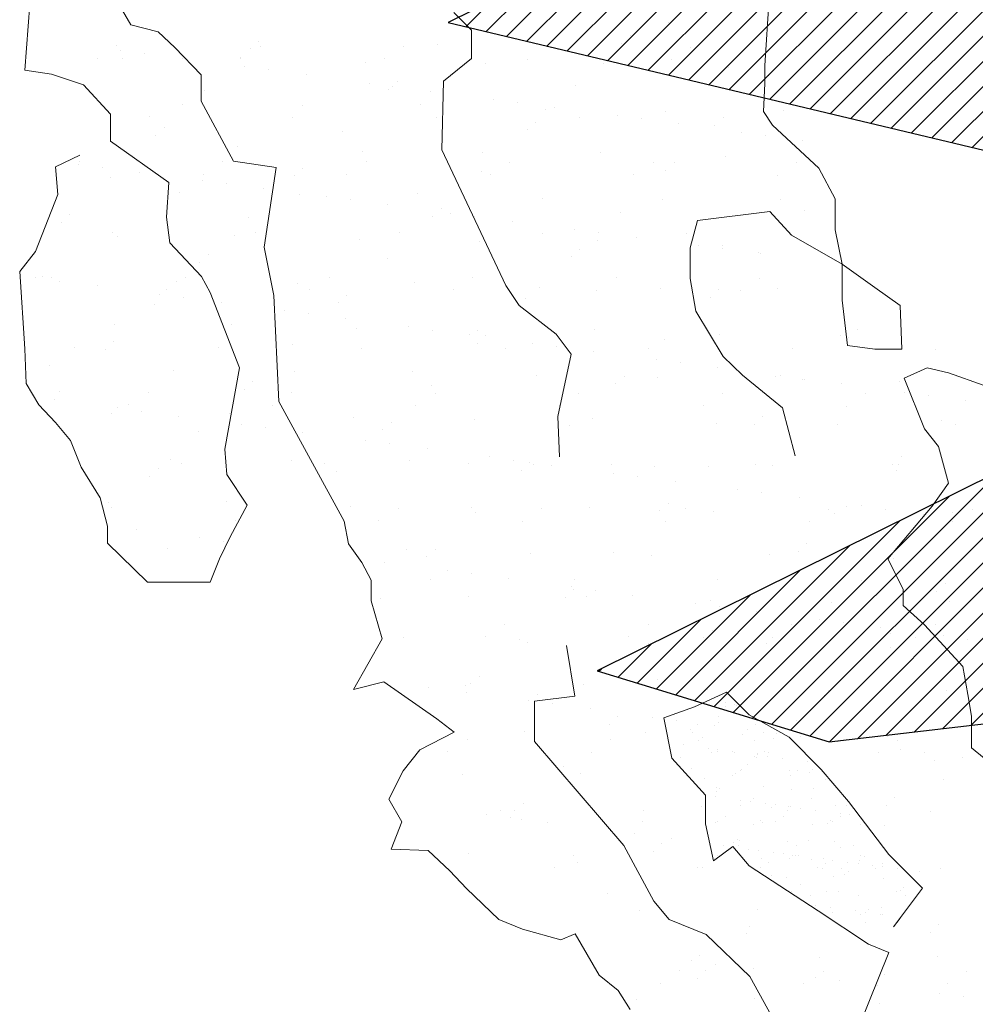
# Model space of a CAD drawing. Units: inches. Extents: x 1986 to 21484, y -1816 to 2016.
# Tile 14 of 85: x 2149.949 to 2158.236, y 1873.899 to 1882.437. Entities that reach past the tile are written whole.
import ezdxf

# ---------------------------------------------------------------- set-up
doc = ezdxf.new("R2010")
doc.units = ezdxf.units.IN
doc.layers.add('L-PLNT', color=84, linetype='Continuous', lineweight=13)
doc.layers.add('vfolhas', color=114, linetype='Continuous', lineweight=5)
doc.layers.add('vfolha2', color=110, linetype='Continuous')
doc.layers.add('vfolhas2', color=102, linetype='Continuous')
pattern_1 = [(45, (-2446.5133113, 50.986076), (-0.004419417382, 0.004419417382), [])]

# ---------------------------------------------------------------- blocks, each defined once
blk = doc.blocks.new('arbusto_PB_verde_grande')
at = {"layer": 'vfolha2'}
h = blk.add_hatch(dxfattribs=at)
h.set_pattern_fill('ANSI31', color=256, scale=0.05, style=0)
h.set_pattern_definition(pattern_1)
h.paths.add_polyline_path([(0.02944, 0.35651), (0.00028, 0.09048), (0.02625, -0.03934), (0.047, 0.06233), (0.06189, 0.09731), (0.09372, 0.26573), (0.09955, 0.43473), (0.08789, 0.61313), (0.0645, 0.72266), (0.04988, 0.6851), (0.0236, 0.51294)])
h.paths.add_polyline_path([(0.30106, 0.43789), (0.14225, 0.24871), (0.26685, 0.30022)])
h.paths.add_polyline_path([(0.37995, 0.22817), (0.23697, 0.15193), (0.18428, 0.09364), (0.11122, 0.04358), (0.02625, -0.03934), (0.28061, 0.04667), (0.36829, 0.07798), (0.46756, 0.11239), (0.61068, 0.19376), (0.71585, 0.27823), (0.55813, 0.25948)])
h.paths.add_polyline_path([(0.56101, -0.29441), (0.72752, -0.32573), (0.59024, -0.2412), (0.42962, -0.15982), (0.02625, -0.03934), (0.14922, -0.14107), (0.18838, -0.16604), (0.41501, -0.24435)])
h.paths.add_polyline_path([(-0.27429, -0.44776), (-0.30352, -0.72628), (-0.23923, -0.64175), (-0.15457, -0.45716), (0.02625, -0.03934), (-0.16328, -0.25376)])
h.paths.add_polyline_path([(-0.51963, -0.24744), (-0.67736, -0.32573), (-0.59558, -0.35072), (-0.40574, -0.32882), (-0.21007, -0.20995), (0.02625, -0.03934), (-0.14874, -0.06595), (-0.31518, -0.09101), (-0.41452, -0.15048)])
h.paths.add_polyline_path([(-0.52546, 0.25007), (-0.70947, 0.24698), (-0.51963, 0.1093), (-0.32979, 0.02167), (-0.07567, -0.0128), (-0.04234, -0.02148), (-0.35024, 0.1312)])
at = {"layer": 'vfolhas'}
h = blk.add_hatch(dxfattribs=at)
h.set_pattern_fill('ANSI31', color=256, scale=0.05, style=0)
h.set_pattern_definition(pattern_1)
h.paths.add_polyline_path([(-0.57219, 0.06233), (-0.7153, 0.10298), (-0.67736, 0.08107), (-0.62769, 0.01536), (-0.56347, -0.04095), (-0.26461, -0.0834), (-0.14874, -0.06595), (-0.10151, -0.05877), (-0.20418, -0.0472), (-0.40279, -0.00339)])
h.paths.add_polyline_path([(-0.56347, -0.04095), (-0.58279, -0.02401), (-0.72992, -0.09726), (-0.4334, -0.1679), (-0.41452, -0.15048), (-0.31518, -0.09101), (-0.26461, -0.0834)])
h.paths.add_polyline_path([(-0.2769, -0.47267), (-0.27429, -0.44776), (-0.16328, -0.25376), (0.02625, -0.03934), (-0.21007, -0.20995), (-0.2672, -0.24466), (-0.36485, -0.35697), (-0.42907, -0.46341), (-0.47586, -0.60425), (-0.37946, -0.57603)])
at = {"layer": 'vfolha2'}
for p, q in [((-0.51963, -0.24744), (-0.67736, -0.32573)), ((-0.67736, -0.32573), (-0.59558, -0.35072)), ((-0.59558, -0.35072), (-0.40574, -0.32882))]:
    blk.add_line(p, q, dxfattribs=at)
at = {"layer": 'vfolhas2'}
for p, q in [((-0.58279, -0.02401), (-0.72992, -0.09726)), ((-0.72992, -0.09726), (-0.4334, -0.1679))]:
    blk.add_line(p, q, dxfattribs=at)
blk = doc.blocks.new('PLANT-SHRUB')
for p, q in [((2156.412, 1882.0396), (2156.4637, 1882.8912)), ((2150.0375, 1882.5728), (2149.9922, 1881.9992)), ((2150.9127, 1882.3924), (2150.8403, 1882.5164)), ((2153.8674, 1882.3451), (2153.7137, 1882.4988)), ((2151.1505, 1882.3304), (2150.9127, 1882.3924)), ((2154.5314, 1882.4284), (2154.5314, 1882.4284)), ((2155.5776, 1882.4151), (2155.5776, 1882.4151)), ((2151.2953, 1882.1961), (2151.1505, 1882.3304)), ((2153.8674, 1882.0994), (2153.8674, 1882.3451)), ((2155.2446, 1882.3002), (2155.2446, 1882.3002)), ((2150.7886, 1882.2088), (2150.7886, 1882.2088)), ((2152.0225, 1882.2512), (2152.0225, 1882.2512)), ((2152.0333, 1882.2065), (2152.0333, 1882.2065)), ((2153.5717, 1882.219), (2153.5717, 1882.219)), ((2155.1709, 1882.2327), (2155.1709, 1882.2327)), ((2150.8264, 1882.1709), (2150.8264, 1882.1709)), ((2151.0345, 1882.1435), (2151.0345, 1882.1435)), ((2151.5228, 1881.9584), (2151.2953, 1882.1961)), ((2151.9488, 1882.1836), (2151.9488, 1882.1836)), ((2153.2779, 1882.2043), (2153.2779, 1882.2043)), ((2154.5225, 1882.202), (2154.5225, 1882.202)), ((2155.7672, 1882.1998), (2155.7672, 1882.1998)), ((2150.6201, 1882.1014), (2150.6201, 1882.1014)), ((2150.843, 1882.101), (2150.843, 1882.101)), ((2151.3594, 1882.1007), (2151.3594, 1882.1007)), ((2151.8647, 1882.0992), (2151.8647, 1882.0992)), ((2151.8654, 1882.1059), (2151.8654, 1882.1059)), ((2152.9448, 1882.0671), (2152.9448, 1882.0671)), ((2153.1094, 1882.0969), (2153.1094, 1882.0969)), ((2153.6229, 1881.9049), (2153.8674, 1882.0994)), ((2153.991, 1882.0537), (2153.991, 1882.0537)), ((2154.354, 1882.0946), (2154.354, 1882.0946)), ((2155.0134, 1882.0586), (2155.0134, 1882.0586)), ((2155.5986, 1882.0924), (2155.5986, 1882.0924)), ((2156.412, 1881.8848), (2156.412, 1882.0396)), ((2149.9922, 1881.9992), (2150.2243, 1881.9644)), ((2150.2243, 1881.9644), (2150.5029, 1881.8716)), ((2151.5228, 1881.7311), (2151.5228, 1881.9584)), ((2151.9022, 1882.0292), (2151.9022, 1882.0292)), ((2152.1103, 1882.0018), (2152.1103, 1882.0018)), ((2152.4352, 1881.9591), (2152.4352, 1881.9591)), ((2156.0929, 1882.0197), (2156.0929, 1882.0197)), ((2156.4461, 1881.9494), (2156.4461, 1881.9494)), ((2150.5029, 1881.8716), (2150.7351, 1881.6164)), ((2152.9781, 1881.8876), (2152.9781, 1881.8876)), ((2153.224, 1881.9004), (2153.224, 1881.9004)), ((2153.6083, 1881.3076), (2153.6229, 1881.9049)), ((2153.6229, 1881.9049), (2153.6229, 1881.9049)), ((2154.7731, 1881.8682), (2154.7731, 1881.8682)), ((2156.3724, 1881.8819), (2156.3724, 1881.8819)), ((2156.3991, 1881.6396), (2156.412, 1881.8848)), ((2151.551, 1881.8191), (2151.551, 1881.8191)), ((2153.1503, 1881.8329), (2153.1503, 1881.8329)), ((2153.1861, 1881.8602), (2153.1861, 1881.8602)), ((2153.511, 1881.8174), (2153.511, 1881.8174)), ((2151.3582, 1881.7057), (2151.3582, 1881.7057)), ((2151.8029, 1881.2105), (2151.5228, 1881.7311)), ((2153.4268, 1881.6972), (2153.4268, 1881.6972)), ((2154.0539, 1881.746), (2154.0539, 1881.746)), ((2154.2619, 1881.7186), (2154.2619, 1881.7186)), ((2150.7351, 1881.6164), (2150.7351, 1881.3844)), ((2152.4044, 1881.6923), (2152.4044, 1881.6923)), ((2154.5063, 1881.6583), (2154.5063, 1881.6583)), ((2154.5868, 1881.6758), (2154.5868, 1881.6758)), ((2155.5524, 1881.645), (2155.5524, 1881.645)), ((2156.4766, 1881.5235), (2156.3991, 1881.6396)), ((2156.5748, 1881.6499), (2156.5748, 1881.6499)), ((2151.0726, 1881.5945), (2151.0726, 1881.5945)), ((2152.3172, 1881.5923), (2152.3172, 1881.5923)), ((2153.5619, 1881.59), (2153.5619, 1881.59)), ((2154.4254, 1881.5496), (2154.4254, 1881.5496)), ((2154.8065, 1881.5877), (2154.8065, 1881.5877)), ((2155.1297, 1881.6043), (2155.1297, 1881.6043)), ((2155.3377, 1881.5769), (2155.3377, 1881.5769)), ((2155.6627, 1881.5342), (2155.6627, 1881.5342)), ((2156.0511, 1881.5855), (2156.0511, 1881.5855)), ((2156.4766, 1881.5235), (2156.8784, 1881.1488)), ((2151.2033, 1881.5005), (2151.2033, 1881.5005)), ((2152.7525, 1881.4683), (2152.7525, 1881.4683)), ((2154.3518, 1881.4821), (2154.3518, 1881.4821)), ((2155.9746, 1881.5174), (2155.9746, 1881.5174)), ((2156.2055, 1881.4627), (2156.2055, 1881.4627)), ((2150.7351, 1881.3844), (2151.2415, 1881.0257)), ((2151.1297, 1881.433), (2151.1297, 1881.433)), ((2156.4136, 1881.4353), (2156.4136, 1881.4353)), ((2156.7385, 1881.3925), (2156.7385, 1881.3925)), ((2150.8178, 1881.331), (2150.8178, 1881.331)), ((2151.8402, 1881.3359), (2151.8402, 1881.3359)), ((2152.9197, 1881.297), (2152.9197, 1881.297)), ((2153.6083, 1881.3076), (2153.6083, 1881.3076)), ((2154.164, 1880.1332), (2153.6083, 1881.3076)), ((2153.9658, 1881.2836), (2153.9658, 1881.2836)), ((2154.9882, 1881.2885), (2154.9882, 1881.2885)), ((2150.2604, 1881.1604), (2150.4713, 1881.2612)), ((2150.4579, 1881.1846), (2150.4579, 1881.1846)), ((2150.4659, 1881.208), (2150.4659, 1881.208)), ((2151.7105, 1881.2057), (2151.7105, 1881.2057)), ((2152.174, 1881.1542), (2151.8029, 1881.2105)), ((2152.9551, 1881.2035), (2152.9551, 1881.2035)), ((2154.1997, 1881.2012), (2154.1997, 1881.2012)), ((2155.4444, 1881.1989), (2155.4444, 1881.1989)), ((2155.6269, 1881.1988), (2155.6269, 1881.1988)), ((2156.0677, 1881.2496), (2156.0677, 1881.2496)), ((2156.689, 1881.1967), (2156.689, 1881.1967)), ((2150.2604, 1881.1604), (2150.2604, 1881.1604)), ((2150.2787, 1880.9221), (2150.2604, 1881.1604)), ((2150.666, 1881.1572), (2150.666, 1881.1572)), ((2150.9909, 1881.1144), (2150.9909, 1881.1144)), ((2151.5419, 1881.0984), (2151.5419, 1881.0984)), ((2152.0694, 1880.4639), (2152.174, 1881.1542)), ((2152.4048, 1881.1497), (2152.4048, 1881.1497)), ((2152.7866, 1881.0961), (2152.7866, 1881.0961)), ((2153.954, 1881.1176), (2153.954, 1881.1176)), ((2155.5532, 1881.1313), (2155.5532, 1881.1313)), ((2156.8784, 1881.1488), (2157.0196, 1880.8823)), ((2150.7319, 1881.0685), (2150.7319, 1881.0685)), ((2151.2415, 1881.0257), (2151.2231, 1880.7233)), ((2151.5337, 1881.0429), (2151.5337, 1881.0429)), ((2151.7418, 1881.0156), (2151.7418, 1881.0156)), ((2152.3311, 1881.0822), (2152.3311, 1881.0822)), ((2154.0312, 1881.0938), (2154.0312, 1881.0938)), ((2155.2758, 1881.0916), (2155.2758, 1881.0916)), ((2156.5205, 1881.0893), (2156.5205, 1881.0893)), ((2151.3331, 1880.9356), (2151.3331, 1880.9356)), ((2152.0667, 1880.9728), (2152.0667, 1880.9728)), ((2153.4016, 1880.9271), (2153.4016, 1880.9271)), ((2150.0861, 1880.4272), (2150.2787, 1880.9221)), ((2152.3792, 1880.9222), (2152.3792, 1880.9222)), ((2152.6096, 1880.9013), (2152.6096, 1880.9013)), ((2152.8176, 1880.8739), (2152.8176, 1880.8739)), ((2154.4811, 1880.8882), (2154.4811, 1880.8882)), ((2155.5273, 1880.8749), (2155.5273, 1880.8749)), ((2156.5497, 1880.8798), (2156.5497, 1880.8798)), ((2157.0196, 1880.8823), (2157.0196, 1880.6157)), ((2153.1425, 1880.8311), (2153.1425, 1880.8311)), ((2153.6062, 1880.799), (2153.6062, 1880.799)), ((2153.6854, 1880.7597), (2153.6854, 1880.7597)), ((2155.1554, 1880.7668), (2155.1554, 1880.7668)), ((2156.4547, 1880.7725), (2155.8271, 1880.6941)), ((2156.643, 1880.5687), (2156.4547, 1880.7725)), ((2156.7547, 1880.7805), (2156.7547, 1880.7805)), ((2150.3105, 1880.6824), (2150.3105, 1880.6824)), ((2150.3841, 1880.7499), (2150.3841, 1880.7499)), ((2151.2231, 1880.7233), (2151.2506, 1880.5033)), ((2151.9333, 1880.7177), (2151.9333, 1880.7177)), ((2153.5326, 1880.7314), (2153.5326, 1880.7314)), ((2153.8934, 1880.7323), (2153.8934, 1880.7323)), ((2154.2184, 1880.6895), (2154.2184, 1880.6895)), ((2155.8271, 1880.6941), (2155.7643, 1880.4589)), ((2150.7498, 1880.5937), (2150.7498, 1880.5937)), ((2151.9944, 1880.5914), (2151.9944, 1880.5914)), ((2153.2391, 1880.5892), (2153.2391, 1880.5892)), ((2154.4837, 1880.5869), (2154.4837, 1880.5869)), ((2154.7612, 1880.618), (2154.7612, 1880.618)), ((2154.9693, 1880.5906), (2154.9693, 1880.5906)), ((2155.7283, 1880.5847), (2155.7283, 1880.5847)), ((2157.0196, 1880.6157), (2157.0823, 1880.3178)), ((2150.7926, 1880.5609), (2150.7926, 1880.5609)), ((2151.2506, 1880.5033), (2151.5258, 1880.2101)), ((2151.815, 1880.5658), (2151.815, 1880.5658)), ((2152.8945, 1880.5269), (2152.8945, 1880.5269)), ((2153.9407, 1880.5135), (2153.9407, 1880.5135)), ((2154.9631, 1880.5184), (2154.9631, 1880.5184)), ((2155.2942, 1880.5479), (2155.2942, 1880.5479)), ((2157.0823, 1880.3178), (2156.643, 1880.5687)), ((2149.9485, 1880.2531), (2150.0861, 1880.4272)), ((2152.1531, 1880.0455), (2152.0694, 1880.4639)), ((2154.8077, 1880.4482), (2154.8077, 1880.4482)), ((2155.7643, 1880.4589), (2155.7643, 1880.1924)), ((2155.837, 1880.4764), (2155.837, 1880.4764)), ((2156.0425, 1880.4795), (2156.0425, 1880.4795)), ((2156.0451, 1880.449), (2156.0451, 1880.449)), ((2156.3569, 1880.416), (2156.3569, 1880.416)), ((2151.5119, 1880.3316), (2151.5119, 1880.3316)), ((2151.5856, 1880.3991), (2151.5856, 1880.3991)), ((2153.1348, 1880.3669), (2153.1348, 1880.3669)), ((2154.734, 1880.3807), (2154.734, 1880.3807)), ((2156.37, 1880.4062), (2156.37, 1880.4062)), ((2149.9485, 1880.2531), (2149.9485, 1880.2531)), ((2149.9944, 1879.5841), (2149.9485, 1880.2531)), ((2157.0823, 1880.0043), (2157.0823, 1880.3178)), ((2157.0823, 1880.3178), (2157.3648, 1880.114)), ((2150.0894, 1880.1983), (2150.0894, 1880.1983)), ((2150.1431, 1880.2072), (2150.1431, 1880.2072)), ((2150.2284, 1880.2044), (2150.2284, 1880.2044)), ((2150.2975, 1880.1709), (2150.2975, 1880.1709)), ((2151.3079, 1880.1655), (2151.3079, 1880.1655)), ((2151.3877, 1880.2049), (2151.3877, 1880.2049)), ((2151.5258, 1880.2101), (2151.5992, 1880.0726)), ((2152.6323, 1880.2026), (2152.6323, 1880.2026)), ((2153.3764, 1880.157), (2153.3764, 1880.157)), ((2153.877, 1880.2004), (2153.877, 1880.2004)), ((2155.1216, 1880.1981), (2155.1216, 1880.1981)), ((2155.7643, 1880.1924), (2155.8114, 1879.9102)), ((2156.3662, 1880.1959), (2156.3662, 1880.1959)), ((2150.6224, 1880.1281), (2150.6224, 1880.1281)), ((2151.2192, 1880.0975), (2151.2192, 1880.0975)), ((2151.5992, 1880.0726), (2151.8562, 1879.4191)), ((2152.3541, 1880.1521), (2152.3541, 1880.1521)), ((2152.4638, 1880.0953), (2152.4638, 1880.0953)), ((2153.7084, 1880.093), (2153.7084, 1880.093)), ((2154.2807, 1879.9584), (2154.164, 1880.1332)), ((2154.4559, 1880.1182), (2154.4559, 1880.1182)), ((2154.9531, 1880.0908), (2154.9531, 1880.0908)), ((2155.5021, 1880.1048), (2155.5021, 1880.1048)), ((2156.0092, 1880.0974), (2156.0092, 1880.0974)), ((2156.1977, 1880.0885), (2156.1977, 1880.0885)), ((2156.5245, 1880.1097), (2156.5245, 1880.1097)), ((2157.3648, 1880.114), (2157.5844, 1879.9572)), ((2151.1653, 1880.0566), (2151.1653, 1880.0566)), ((2151.3733, 1880.0293), (2151.3733, 1880.0293)), ((2151.6982, 1879.9865), (2151.6982, 1879.9865)), ((2152.1531, 1880.0455), (2152.1531, 1880.0455)), ((2152.195, 1879.125), (2152.1531, 1880.0455)), ((2152.7871, 1880.0483), (2152.7871, 1880.0483)), ((2154.3362, 1880.0161), (2154.3362, 1880.0161)), ((2155.9355, 1880.0299), (2155.9355, 1880.0299)), ((2157.1294, 1879.6123), (2157.0823, 1880.0043)), ((2151.1141, 1879.9671), (2151.1141, 1879.9671)), ((2152.2411, 1879.915), (2152.2411, 1879.915)), ((2152.7134, 1879.9808), (2152.7134, 1879.9808)), ((2154.6015, 1879.7107), (2154.2807, 1879.9584)), ((2155.8114, 1879.9102), (2156.0496, 1879.5165)), ((2157.5844, 1879.9572), (2157.6001, 1879.5809)), ((2157.5844, 1879.9572), (2157.5844, 1879.9572)), ((2152.4491, 1879.8876), (2152.4491, 1879.8876)), ((2152.774, 1879.8448), (2152.774, 1879.8448)), ((2150.7674, 1879.7908), (2150.7674, 1879.7908)), ((2151.7898, 1879.7957), (2151.7898, 1879.7957)), ((2152.8693, 1879.7568), (2152.8693, 1879.7568)), ((2153.3169, 1879.7734), (2153.3169, 1879.7734)), ((2153.5249, 1879.746), (2153.5249, 1879.746)), ((2153.9155, 1879.7434), (2153.9155, 1879.7434)), ((2154.9379, 1879.7483), (2154.9379, 1879.7483)), ((2157.2106, 1879.7466), (2157.2106, 1879.7466)), ((2150.7664, 1879.6485), (2150.7664, 1879.6485)), ((2153.8499, 1879.7032), (2153.8499, 1879.7032)), ((2153.9885, 1879.6975), (2153.9885, 1879.6975)), ((2154.7327, 1879.5359), (2154.6015, 1879.7107)), ((2155.5377, 1879.6654), (2155.5377, 1879.6654)), ((2156.0173, 1879.7094), (2156.0173, 1879.7094)), ((2157.0635, 1879.6961), (2157.0635, 1879.6961)), ((2157.137, 1879.6791), (2157.137, 1879.6791)), ((2150.0035, 1879.2817), (2149.9944, 1879.5841)), ((2150.427, 1879.5929), (2150.427, 1879.5929)), ((2150.6928, 1879.581), (2150.6928, 1879.581)), ((2151.6717, 1879.5906), (2151.6717, 1879.5906)), ((2152.3156, 1879.6163), (2152.3156, 1879.6163)), ((2152.9163, 1879.5884), (2152.9163, 1879.5884)), ((2153.9149, 1879.63), (2153.9149, 1879.63)), ((2154.1609, 1879.5861), (2154.1609, 1879.5861)), ((2154.3927, 1879.6317), (2154.3927, 1879.6317)), ((2154.6008, 1879.6044), (2154.6008, 1879.6044)), ((2154.9257, 1879.5616), (2154.9257, 1879.5616)), ((2155.4056, 1879.5838), (2155.4056, 1879.5838)), ((2156.6502, 1879.5816), (2156.6502, 1879.5816)), ((2157.3648, 1879.5809), (2157.1294, 1879.6123)), ((2157.6001, 1879.5809), (2157.3648, 1879.5809)), ((2157.8948, 1879.5793), (2157.8948, 1879.5793)), ((2154.6161, 1878.9968), (2154.7327, 1879.5359)), ((2155.4685, 1879.4901), (2155.4685, 1879.4901)), ((2156.0496, 1879.5165), (2156.2178, 1879.3557)), ((2150.2032, 1879.4343), (2150.2032, 1879.4343)), ((2151.2827, 1879.3954), (2151.2827, 1879.3954)), ((2151.8562, 1879.4191), (2151.7278, 1878.7135)), ((2155.6766, 1879.4627), (2155.6766, 1879.4627)), ((2156.0015, 1879.4199), (2156.0015, 1879.4199)), ((2157.6195, 1879.3297), (2157.8177, 1879.4177)), ((2157.8177, 1879.4177), (2158.0049, 1879.3737)), ((2152.3289, 1879.382), (2152.3289, 1879.382)), ((2153.3513, 1879.3869), (2153.3513, 1879.3869)), ((2154.4307, 1879.3481), (2154.4307, 1879.3481)), ((2155.19, 1879.3468), (2155.19, 1879.3468)), ((2155.4769, 1879.3347), (2155.4769, 1879.3347)), ((2156.2178, 1879.3557), (2156.5647, 1879.0723)), ((2156.4993, 1879.3396), (2156.4993, 1879.3396)), ((2156.5444, 1879.3485), (2156.5444, 1879.3485)), ((2156.7392, 1879.3146), (2156.7392, 1879.3146)), ((2156.7524, 1879.3211), (2156.7524, 1879.3211)), ((2157.7956, 1878.8896), (2157.6195, 1879.3297)), ((2158.0049, 1879.3737), (2158.3132, 1879.2637)), ((2150.1136, 1879.0984), (2150.0035, 1879.2817)), ((2151.8942, 1879.2302), (2151.8942, 1879.2302)), ((2151.9679, 1879.2977), (2151.9679, 1879.2977)), ((2153.5171, 1879.2655), (2153.5171, 1879.2655)), ((2155.1163, 1879.2792), (2155.1163, 1879.2792)), ((2157.0773, 1879.2783), (2157.0773, 1879.2783)), ((2157.5788, 1879.3007), (2157.5788, 1879.3007)), ((2150.2539, 1879.1418), (2150.2539, 1879.1418)), ((2150.295, 1879.2164), (2150.295, 1879.2164)), ((2151.0649, 1879.2041), (2151.0649, 1879.2041)), ((2152.3095, 1879.2018), (2152.3095, 1879.2018)), ((2153.5542, 1879.1996), (2153.5542, 1879.1996)), ((2154.7988, 1879.1973), (2154.7988, 1879.1973)), ((2156.0434, 1879.195), (2156.0434, 1879.195)), ((2157.2881, 1879.1928), (2157.2881, 1879.1928)), ((2157.6202, 1879.2068), (2157.6202, 1879.2068)), ((2157.8282, 1879.1794), (2157.8282, 1879.1794)), ((2158.1532, 1879.1367), (2158.1532, 1879.1367)), ((2150.2604, 1878.9426), (2150.1136, 1879.0984)), ((2150.7968, 1879.0703), (2150.7968, 1879.0703)), ((2150.8964, 1879.0967), (2150.8964, 1879.0967)), ((2152.141, 1879.0945), (2152.141, 1879.0945)), ((2152.195, 1879.125), (2152.195, 1879.125)), ((2152.7632, 1878.0871), (2152.195, 1879.125)), ((2153.3856, 1879.0922), (2153.3856, 1879.0922)), ((2154.6303, 1879.0899), (2154.6303, 1879.0899)), ((2155.8749, 1879.0877), (2155.8749, 1879.0877)), ((2156.5647, 1879.0723), (2156.6744, 1878.6559)), ((2157.1195, 1879.0854), (2157.1195, 1879.0854)), ((2150.7423, 1879.0207), (2150.7423, 1879.0207)), ((2151.0048, 1879.043), (2151.0048, 1879.043)), ((2151.3297, 1879.0002), (2151.3297, 1879.0002)), ((2151.7647, 1879.0256), (2151.7647, 1879.0256)), ((2152.8441, 1878.9867), (2152.8441, 1878.9867)), ((2153.8903, 1878.9733), (2153.8903, 1878.9733)), ((2154.6306, 1878.6471), (2154.6161, 1878.9968)), ((2154.9127, 1878.9782), (2154.9127, 1878.9782)), ((2156.3915, 1878.996), (2156.3915, 1878.996)), ((2157.9406, 1878.9638), (2157.9406, 1878.9638)), ((2150.3888, 1878.7868), (2150.2604, 1878.9426)), ((2151.8726, 1878.9287), (2151.8726, 1878.9287)), ((2152.0806, 1878.9013), (2152.0806, 1878.9013)), ((2153.0957, 1878.8794), (2153.0957, 1878.8794)), ((2153.1694, 1878.9469), (2153.1694, 1878.9469)), ((2154.7185, 1878.9147), (2154.7185, 1878.9147)), ((2155.9922, 1878.9393), (2155.9922, 1878.9393)), ((2156.3178, 1878.9285), (2156.3178, 1878.9285)), ((2157.0383, 1878.926), (2157.0383, 1878.926)), ((2157.9168, 1878.7356), (2157.7956, 1878.8896)), ((2158.0607, 1878.9309), (2158.0607, 1878.9309)), ((2151.4964, 1878.8657), (2151.4964, 1878.8657)), ((2152.4055, 1878.8585), (2152.4055, 1878.8585)), ((2150.4805, 1878.5577), (2150.3888, 1878.7868)), ((2151.7278, 1878.7135), (2151.7462, 1878.4935)), ((2152.9484, 1878.7871), (2152.9484, 1878.7871)), ((2153.1564, 1878.7597), (2153.1564, 1878.7597)), ((2153.4814, 1878.7169), (2153.4814, 1878.7169)), ((2158.0049, 1878.4165), (2157.9168, 1878.7356)), ((2151.2575, 1878.6253), (2151.2575, 1878.6253)), ((2154.0242, 1878.6454), (2154.0242, 1878.6454)), ((2157.5929, 1878.6452), (2157.5929, 1878.6452)), ((2150.6456, 1878.2919), (2150.4805, 1878.5577)), ((2151.1487, 1878.547), (2151.1487, 1878.547)), ((2151.3489, 1878.5898), (2151.3489, 1878.5898)), ((2152.3037, 1878.6119), (2152.3037, 1878.6119)), ((2152.5935, 1878.5876), (2152.5935, 1878.5876)), ((2153.3261, 1878.6169), (2153.3261, 1878.6169)), ((2153.8381, 1878.5853), (2153.8381, 1878.5853)), ((2154.2323, 1878.6181), (2154.2323, 1878.6181)), ((2154.3708, 1878.5961), (2154.3708, 1878.5961)), ((2154.4056, 1878.578), (2154.4056, 1878.578)), ((2154.5572, 1878.5753), (2154.5572, 1878.5753)), ((2155.0828, 1878.583), (2155.0828, 1878.583)), ((2155.4517, 1878.5646), (2155.4517, 1878.5646)), ((2155.92, 1878.5639), (2155.92, 1878.5639)), ((2156.3274, 1878.5808), (2156.3274, 1878.5808)), ((2156.4741, 1878.5695), (2156.4741, 1878.5695)), ((2157.5193, 1878.5777), (2157.5193, 1878.5777)), ((2157.572, 1878.5785), (2157.572, 1878.5785)), ((2151.075, 1878.4795), (2151.075, 1878.4795)), ((2151.7462, 1878.4935), (2151.9204, 1878.2277)), ((2152.6979, 1878.5149), (2152.6979, 1878.5149)), ((2154.2971, 1878.5286), (2154.2971, 1878.5286)), ((2155.1001, 1878.5038), (2155.1001, 1878.5038)), ((2155.3081, 1878.4764), (2155.3081, 1878.4764)), ((2157.5536, 1878.5306), (2157.5536, 1878.5306)), ((2155.633, 1878.4336), (2155.633, 1878.4336)), ((2157.8617, 1878.2184), (2158.0049, 1878.4165)), ((2158.0049, 1878.4165), (2158.0049, 1878.4165)), ((2150.7098, 1878.0444), (2150.6456, 1878.2919)), ((2156.1759, 1878.3622), (2156.1759, 1878.3622)), ((2156.3839, 1878.3348), (2156.3839, 1878.3348)), ((2156.7088, 1878.292), (2156.7088, 1878.292)), ((2150.7171, 1878.2506), (2150.7171, 1878.2506)), ((2150.7421, 1878.2033), (2150.7421, 1878.2033)), ((2151.7395, 1878.2555), (2151.7395, 1878.2555)), ((2151.9204, 1878.2277), (2151.7737, 1877.9528)), ((2152.819, 1878.2166), (2152.819, 1878.2166)), ((2153.2314, 1878.1988), (2153.2314, 1878.1988)), ((2153.8651, 1878.2032), (2153.8651, 1878.2032)), ((2154.476, 1878.1965), (2154.476, 1878.1965)), ((2154.8875, 1878.2081), (2154.8875, 1878.2081)), ((2155.5723, 1878.2453), (2155.5723, 1878.2453)), ((2155.7207, 1878.1942), (2155.7207, 1878.1942)), ((2157.1215, 1878.2132), (2157.1215, 1878.2132)), ((2157.2517, 1878.2205), (2157.2517, 1878.2205)), ((2157.4597, 1878.1932), (2157.4597, 1878.1932)), ((2157.4779, 1877.7629), (2157.8617, 1878.2184)), ((2153.8993, 1878.1641), (2153.8993, 1878.1641)), ((2155.4986, 1878.1778), (2155.4986, 1878.1778)), ((2155.967, 1878.1692), (2155.967, 1878.1692)), ((2156.9653, 1878.192), (2156.9653, 1878.192)), ((2157.0132, 1878.1559), (2157.0132, 1878.1559)), ((2157.7847, 1878.1504), (2157.7847, 1878.1504)), ((2158.0356, 1878.1608), (2158.0356, 1878.1608)), ((2158.2099, 1878.1897), (2158.2099, 1878.1897)), ((2150.7098, 1877.8978), (2150.7098, 1878.0444)), ((2151.8182, 1878.0936), (2151.8182, 1878.0936)), ((2152.7996, 1877.8907), (2152.7632, 1878.0871)), ((2153.0629, 1878.0914), (2153.0629, 1878.0914)), ((2154.3075, 1878.0891), (2154.3075, 1878.0891)), ((2155.5521, 1878.0869), (2155.5521, 1878.0869)), ((2156.7968, 1878.0846), (2156.7968, 1878.0846)), ((2158.0414, 1878.0823), (2158.0414, 1878.0823)), ((2150.9612, 1878.0139), (2150.9612, 1878.0139)), ((2151.5041, 1877.9424), (2151.5041, 1877.9424)), ((2151.7737, 1877.9528), (2151.682, 1877.7603)), ((2151.0583, 1877.5587), (2150.7098, 1877.8978)), ((2151.2323, 1877.8552), (2151.2323, 1877.8552)), ((2151.7121, 1877.915), (2151.7121, 1877.915)), ((2152.9161, 1877.7307), (2152.7996, 1877.8907)), ((2156.7737, 1877.8946), (2156.7737, 1877.8946)), ((2153.3009, 1877.8468), (2153.3009, 1877.8468)), ((2153.478, 1877.778), (2153.478, 1877.778)), ((2153.5516, 1877.8455), (2153.5516, 1877.8455)), ((2154.3804, 1877.8079), (2154.3804, 1877.8079)), ((2155.1008, 1877.8133), (2155.1008, 1877.8133)), ((2155.4266, 1877.7945), (2155.4266, 1877.7945)), ((2156.449, 1877.7994), (2156.449, 1877.7994)), ((2156.7001, 1877.827), (2156.7001, 1877.827)), ((2151.682, 1877.7603), (2151.5994, 1877.5587)), ((2152.9962, 1877.5779), (2152.9161, 1877.7307)), ((2153.1129, 1877.7306), (2153.1129, 1877.7306)), ((2157.61, 1877.4988), (2157.4779, 1877.7629)), ((2157.5284, 1877.7605), (2157.5284, 1877.7605)), ((2153.6557, 1877.6591), (2153.6557, 1877.6591)), ((2153.8638, 1877.6318), (2153.8638, 1877.6318)), ((2151.0583, 1877.5587), (2151.0583, 1877.5587)), ((2151.5994, 1877.5587), (2151.0583, 1877.5587)), ((2152.9962, 1877.3961), (2152.9962, 1877.5779)), ((2153.5154, 1877.5845), (2153.5154, 1877.5845)), ((2154.1887, 1877.589), (2154.1887, 1877.589)), ((2154.7316, 1877.5175), (2154.7316, 1877.5175)), ((2154.76, 1877.5822), (2154.76, 1877.5822)), ((2156.0046, 1877.58), (2156.0046, 1877.58)), ((2157.2493, 1877.5777), (2157.2493, 1877.5777)), ((2157.9752, 1877.5438), (2157.9752, 1877.5438)), ((2153.84, 1877.4331), (2153.84, 1877.4331)), ((2154.6794, 1877.4272), (2154.6794, 1877.4272)), ((2154.7531, 1877.4947), (2154.7531, 1877.4947)), ((2154.8623, 1877.438), (2154.8623, 1877.438)), ((2154.9396, 1877.4901), (2154.9396, 1877.4901)), ((2155.2645, 1877.4473), (2155.2645, 1877.4473)), ((2156.3023, 1877.4625), (2156.3023, 1877.4625)), ((2157.61, 1877.3558), (2157.61, 1877.4988)), ((2157.9015, 1877.4763), (2157.9015, 1877.4763)), ((2153.0908, 1877.0688), (2152.9962, 1877.3961)), ((2153.0802, 1877.4135), (2153.0802, 1877.4135)), ((2155.8074, 1877.3759), (2155.8074, 1877.3759)), ((2155.9418, 1877.3992), (2155.9418, 1877.3992)), ((2156.0154, 1877.3485), (2156.0154, 1877.3485)), ((2156.988, 1877.3858), (2156.988, 1877.3858)), ((2157.7972, 1877.1907), (2157.61, 1877.3558)), ((2158.0104, 1877.3907), (2158.0104, 1877.3907)), ((2156.3403, 1877.3057), (2156.3403, 1877.3057)), ((2154.1532, 1877.1957), (2154.1532, 1877.1957)), ((2155.3979, 1877.1934), (2155.3979, 1877.1934)), ((2156.6425, 1877.1912), (2156.6425, 1877.1912)), ((2156.8832, 1877.2342), (2156.8832, 1877.2342)), ((2157.0912, 1877.2069), (2157.0912, 1877.2069)), ((2158.1275, 1876.8277), (2157.7972, 1877.1907)), ((2157.8871, 1877.1889), (2157.8871, 1877.1889)), ((2153.9847, 1877.0883), (2153.9847, 1877.0883)), ((2155.2293, 1877.086), (2155.2293, 1877.086)), ((2155.9546, 1877.1439), (2155.9546, 1877.1439)), ((2156.474, 1877.0838), (2156.474, 1877.0838)), ((2157.4162, 1877.1641), (2157.4162, 1877.1641)), ((2157.5037, 1877.1117), (2157.5037, 1877.1117)), ((2157.959, 1877.0926), (2157.959, 1877.0926)), ((2152.8445, 1876.6296), (2153.0908, 1877.0688)), ((2153.2757, 1877.0767), (2153.2757, 1877.0767)), ((2154.2816, 1877.0627), (2154.2816, 1877.0627)), ((2154.3552, 1877.0378), (2154.3552, 1877.0378)), ((2154.7639, 1876.5721), (2154.691, 1877.0092)), ((2155.4014, 1877.0244), (2155.4014, 1877.0244)), ((2155.8809, 1877.0764), (2155.8809, 1877.0764)), ((2156.4238, 1877.0293), (2156.4238, 1877.0293)), ((2157.7186, 1877.0815), (2157.7186, 1877.0815)), ((2158.1671, 1877.0652), (2158.1671, 1877.0652)), ((2157.5032, 1876.9904), (2157.5032, 1876.9904)), ((2158.1275, 1876.8277), (2158.1275, 1876.8277)), ((2158.1716, 1876.5856), (2158.1275, 1876.8277)), ((2153.9339, 1876.7441), (2153.9339, 1876.7441)), ((2157.156, 1876.7931), (2157.156, 1876.7931)), ((2153.1065, 1876.695), (2152.8445, 1876.6296)), ((2153.5651, 1876.375), (2153.1065, 1876.695)), ((2153.8148, 1876.663), (2153.8148, 1876.663)), ((2153.8603, 1876.6766), (2153.8603, 1876.6766)), ((2154.8372, 1876.6679), (2154.8372, 1876.6679)), ((2155.4831, 1876.7119), (2155.4831, 1876.7119)), ((2157.0824, 1876.7256), (2157.0824, 1876.7256)), ((2153.4953, 1876.6455), (2153.4953, 1876.6455)), ((2153.8202, 1876.6027), (2153.8202, 1876.6027)), ((2154.4139, 1876.5284), (2154.7639, 1876.5721)), ((2154.4372, 1876.5814), (2154.4372, 1876.5814)), ((2155.6818, 1876.5791), (2155.6818, 1876.5791)), ((2155.8, 1876.4792), (2156.0787, 1876.6045)), ((2155.9166, 1876.6291), (2155.9166, 1876.6291)), ((2156.0787, 1876.6045), (2156.2738, 1876.4095)), ((2156.9265, 1876.5769), (2156.9265, 1876.5769)), ((2156.9628, 1876.6157), (2156.9628, 1876.6157)), ((2157.9852, 1876.6206), (2157.9852, 1876.6206)), ((2158.1711, 1876.5746), (2158.1711, 1876.5746)), ((2158.2046, 1876.3985), (2158.1716, 1876.5856)), ((2154.3631, 1876.5312), (2154.3631, 1876.5312)), ((2154.4139, 1876.1787), (2154.4139, 1876.5284)), ((2154.5711, 1876.5038), (2154.5711, 1876.5038)), ((2156.0677, 1876.5138), (2156.0677, 1876.5138)), ((2156.1509, 1876.5028), (2156.1509, 1876.5028)), ((2156.1649, 1876.4857), (2156.1649, 1876.4857)), ((2154.896, 1876.4611), (2154.896, 1876.4611)), ((2155.5352, 1876.3817), (2155.8, 1876.4792)), ((2155.5943, 1876.4028), (2155.5943, 1876.4028)), ((2156.074, 1876.482), (2156.074, 1876.482)), ((2156.2738, 1876.4095), (2156.6222, 1876.2146)), ((2153.5651, 1876.375), (2153.5651, 1876.375)), ((2153.718, 1876.2586), (2153.5651, 1876.375)), ((2155.0617, 1876.3258), (2155.0617, 1876.3258)), ((2155.1354, 1876.3933), (2155.1354, 1876.3933)), ((2155.4389, 1876.3896), (2155.4389, 1876.3896)), ((2155.6048, 1876.0336), (2155.5352, 1876.3817)), ((2155.6469, 1876.3622), (2155.6469, 1876.3622)), ((2155.8313, 1876.3274), (2155.8313, 1876.3274)), ((2155.9718, 1876.3194), (2155.9718, 1876.3194)), ((2156.0058, 1876.3399), (2156.0058, 1876.3399)), ((2156.0128, 1876.3974), (2156.0128, 1876.3974)), ((2156.3292, 1876.3265), (2156.3292, 1876.3265)), ((2156.6846, 1876.3611), (2156.6846, 1876.3611)), ((2158.2046, 1876.1235), (2158.2046, 1876.3985)), ((2153.4195, 1876.1058), (2153.718, 1876.2586)), ((2154.33, 1876.2677), (2154.33, 1876.2677)), ((2155.3762, 1876.2543), (2155.3762, 1876.2543)), ((2155.7639, 1876.2845), (2155.7639, 1876.2845)), ((2155.7871, 1876.2548), (2155.7871, 1876.2548)), ((2156.2189, 1876.2393), (2156.2189, 1876.2393)), ((2156.2618, 1876.2836), (2156.2618, 1876.2836)), ((2156.3986, 1876.2592), (2156.3986, 1876.2592)), ((2156.5147, 1876.2479), (2156.5147, 1876.2479)), ((2153.8305, 1876.1949), (2153.8305, 1876.1949)), ((2155.1868, 1875.2753), (2154.4139, 1876.1787)), ((2155.0751, 1876.1926), (2155.0751, 1876.1926)), ((2155.7032, 1876.1478), (2155.7032, 1876.1478)), ((2155.8373, 1876.1855), (2155.8373, 1876.1855)), ((2155.8667, 1876.2125), (2155.8667, 1876.2125)), ((2156.3197, 1876.1903), (2156.3197, 1876.1903)), ((2156.4864, 1876.1996), (2156.4864, 1876.1996)), ((2156.6222, 1876.2146), (2156.9009, 1875.9361)), ((2156.6222, 1876.2146), (2156.6222, 1876.2146)), ((2156.7227, 1876.2206), (2156.7227, 1876.2206)), ((2157.0477, 1876.1778), (2157.0477, 1876.1778)), ((2157.4781, 1876.2203), (2157.4781, 1876.2203)), ((2157.5644, 1876.1881), (2157.5644, 1876.1881)), ((2153.274, 1875.924), (2153.4195, 1876.1058)), ((2153.6619, 1876.0875), (2153.6619, 1876.0875)), ((2154.9065, 1876.0852), (2154.9065, 1876.0852)), ((2155.9203, 1876.1192), (2155.9203, 1876.1192)), ((2155.9449, 1876.0817), (2155.9449, 1876.0817)), ((2156.0027, 1876.0894), (2156.0027, 1876.0894)), ((2156.0035, 1876.1083), (2156.0035, 1876.1083)), ((2156.1335, 1876.0912), (2156.1335, 1876.0912)), ((2156.1512, 1876.083), (2156.1512, 1876.083)), ((2156.3473, 1876.0721), (2156.3473, 1876.0721)), ((2156.3507, 1876.0626), (2156.3507, 1876.0626)), ((2156.4116, 1876.0913), (2156.4116, 1876.0913)), ((2156.4428, 1876.0808), (2156.4428, 1876.0808)), ((2157.3958, 1876.0807), (2157.3958, 1876.0807)), ((2157.5905, 1876.1063), (2157.5905, 1876.1063)), ((2157.7986, 1876.0789), (2157.7986, 1876.0789)), ((2158.3918, 1875.9694), (2158.2046, 1876.1235)), ((2155.6048, 1876.0336), (2155.6048, 1876.0336)), ((2155.8975, 1875.7133), (2155.6048, 1876.0336)), ((2155.6781, 1876.0396), (2155.6781, 1876.0396)), ((2156.2632, 1875.975), (2156.2632, 1875.975)), ((2156.3178, 1876.0451), (2156.3178, 1876.0451)), ((2156.3368, 1876.0425), (2156.3368, 1876.0425)), ((2156.4339, 1876.0516), (2156.4339, 1876.0516)), ((2156.5638, 1876.0345), (2156.5638, 1876.0345)), ((2156.781, 1876.0059), (2156.781, 1876.0059)), ((2157.886, 1876.0103), (2157.886, 1876.0103)), ((2158.1235, 1876.0361), (2158.1235, 1876.0361)), ((2153.1499, 1875.678), (2153.274, 1875.924)), ((2153.7896, 1875.8929), (2153.7896, 1875.8929)), ((2154.6639, 1875.9613), (2154.6639, 1875.9613)), ((2154.812, 1875.8979), (2154.812, 1875.8979)), ((2155.7022, 1875.9271), (2155.7022, 1875.9271)), ((2155.777, 1875.9468), (2155.777, 1875.9468)), ((2156.1587, 1875.8993), (2156.1587, 1875.8993)), ((2156.2001, 1875.9262), (2156.2001, 1875.9262)), ((2156.2088, 1875.9312), (2156.2088, 1875.9312)), ((2156.6273, 1875.9259), (2156.6273, 1875.9259)), ((2156.6979, 1875.9253), (2156.6979, 1875.9253)), ((2156.7984, 1875.9048), (2156.7984, 1875.9048)), ((2156.8279, 1875.9318), (2156.8279, 1875.9318)), ((2156.9009, 1875.9361), (2157.1379, 1875.6576)), ((2155.8915, 1875.859), (2155.8915, 1875.859)), ((2156.1327, 1875.8833), (2156.1327, 1875.8833)), ((2156.6305, 1875.8823), (2156.6305, 1875.8823)), ((2156.9376, 1875.8456), (2156.9376, 1875.8456)), ((2157.96, 1875.8505), (2157.96, 1875.8505)), ((2155.9902, 1875.7449), (2155.9902, 1875.7449)), ((2155.9926, 1875.7813), (2155.9926, 1875.7813)), ((2156.0196, 1875.7719), (2156.0196, 1875.7719)), ((2156.4016, 1875.7833), (2156.4016, 1875.7833)), ((2156.6393, 1875.759), (2156.6393, 1875.759)), ((2156.8334, 1875.7678), (2156.8334, 1875.7678)), ((2153.1499, 1875.678), (2153.1499, 1875.678)), ((2153.2639, 1875.4814), (2153.1499, 1875.678)), ((2154.3162, 1875.6426), (2154.3162, 1875.6426)), ((2155.8975, 1875.4626), (2155.8975, 1875.7133)), ((2155.9861, 1875.6967), (2155.9861, 1875.6967)), ((2156.2033, 1875.6681), (2156.2033, 1875.6681)), ((2156.2865, 1875.6571), (2156.2865, 1875.6571)), ((2156.3137, 1875.6805), (2156.3137, 1875.6805)), ((2156.4165, 1875.64), (2156.4165, 1875.64)), ((2156.5002, 1875.6316), (2156.5002, 1875.6316)), ((2156.8115, 1875.6796), (2156.8115, 1875.6796)), ((2157.1379, 1875.6576), (2157.4863, 1875.198)), ((2157.5383, 1875.6917), (2157.5383, 1875.6917)), ((2154.1144, 1875.5806), (2154.1144, 1875.5806)), ((2154.2425, 1875.5751), (2154.2425, 1875.5751)), ((2155.359, 1875.5783), (2155.359, 1875.5783)), ((2155.8654, 1875.6105), (2155.8654, 1875.6105)), ((2156.1987, 1875.6232), (2156.1987, 1875.6232)), ((2156.4708, 1875.6046), (2156.4708, 1875.6046)), ((2156.6037, 1875.5761), (2156.6037, 1875.5761)), ((2156.6172, 1875.6179), (2156.6172, 1875.6179)), ((2156.6336, 1875.6114), (2156.6336, 1875.6114)), ((2156.7168, 1875.6005), (2156.7168, 1875.6005)), ((2156.8468, 1875.5833), (2156.8468, 1875.5833)), ((2157.0261, 1875.6198), (2157.0261, 1875.6198)), ((2157.0639, 1875.5548), (2157.0639, 1875.5548)), ((2157.1199, 1875.6187), (2157.1199, 1875.6187)), ((2157.4646, 1875.6242), (2157.4646, 1875.6242)), ((2157.8483, 1875.5738), (2157.8483, 1875.5738)), ((2153.1706, 1875.2434), (2153.2639, 1875.4814)), ((2153.2639, 1875.4814), (2153.2639, 1875.4814)), ((2153.9946, 1875.5449), (2153.9946, 1875.5449)), ((2154.2026, 1875.5175), (2154.2026, 1875.5175)), ((2154.3049, 1875.4976), (2154.3049, 1875.4976)), ((2154.5275, 1875.4748), (2154.5275, 1875.4748)), ((2155.351, 1875.4842), (2155.351, 1875.4842)), ((2155.9672, 1875.1423), (2155.8975, 1875.4626)), ((2155.9825, 1875.4733), (2155.9825, 1875.4733)), ((2156.0035, 1875.4829), (2156.0035, 1875.4829)), ((2156.071, 1875.5259), (2156.071, 1875.5259)), ((2156.3734, 1875.4891), (2156.3734, 1875.4891)), ((2156.3915, 1875.4753), (2156.3915, 1875.4753)), ((2156.5014, 1875.482), (2156.5014, 1875.482)), ((2156.5688, 1875.525), (2156.5688, 1875.525)), ((2156.9513, 1875.4643), (2156.9513, 1875.4643)), ((2156.9808, 1875.4913), (2156.9808, 1875.4913)), ((2156.9992, 1875.4811), (2156.9992, 1875.4811)), ((2157.0667, 1875.5241), (2157.0667, 1875.5241)), ((2157.1471, 1875.5438), (2157.1471, 1875.5438)), ((2155.0704, 1875.4033), (2155.0704, 1875.4033)), ((2155.2784, 1875.3759), (2155.2784, 1875.3759)), ((2156.3116, 1875.4588), (2156.3116, 1875.4588)), ((2156.8233, 1875.4597), (2156.8233, 1875.4597)), ((2157.2418, 1875.4544), (2157.2418, 1875.4544)), ((2157.4529, 1875.4502), (2157.4529, 1875.4502)), ((2155.5177, 1875.2919), (2155.5177, 1875.2919)), ((2155.6033, 1875.3331), (2155.6033, 1875.3331)), ((2156.1431, 1875.3043), (2156.1431, 1875.3043)), ((2156.1726, 1875.3313), (2156.1726, 1875.3313)), ((2156.1886, 1875.3152), (2156.1886, 1875.3152)), ((2156.6071, 1875.3098), (2156.6071, 1875.3098)), ((2156.7922, 1875.3185), (2156.7922, 1875.3185)), ((2157.0161, 1875.3118), (2157.0161, 1875.3118)), ((2153.4917, 1875.233), (2153.1706, 1875.2434)), ((2153.6782, 1875.0571), (2153.4917, 1875.233)), ((2153.8447, 1875.2106), (2153.8447, 1875.2106)), ((2155.4492, 1874.7945), (2155.1868, 1875.2753)), ((2155.444, 1875.2243), (2155.444, 1875.2243)), ((2156.1344, 1875.2676), (2155.9672, 1875.1423)), ((2156.0559, 1875.2735), (2156.0559, 1875.2735)), ((2156.2738, 1875.1005), (2156.1344, 1875.2676)), ((2156.1391, 1875.2626), (2156.1391, 1875.2626)), ((2156.1462, 1875.2617), (2156.1462, 1875.2617)), ((2156.1845, 1875.2802), (2156.1845, 1875.2802)), ((2156.2691, 1875.2455), (2156.2691, 1875.2455)), ((2156.3542, 1875.2343), (2156.3542, 1875.2343)), ((2156.4862, 1875.2169), (2156.4862, 1875.2169)), ((2156.5694, 1875.2059), (2156.5694, 1875.2059)), ((2156.6824, 1875.2793), (2156.6824, 1875.2793)), ((2157.0668, 1875.2597), (2157.0668, 1875.2597)), ((2157.1802, 1875.2784), (2157.1802, 1875.2784)), ((2154.7523, 1875.1918), (2154.7523, 1875.1918)), ((2154.7868, 1875.1278), (2154.7868, 1875.1278)), ((2155.9672, 1875.1423), (2155.9672, 1875.1423)), ((2155.9725, 1875.1653), (2155.9725, 1875.1653)), ((2155.984, 1875.1585), (2155.984, 1875.1585)), ((2155.9969, 1875.1895), (2155.9969, 1875.1895)), ((2156.3814, 1875.1672), (2156.3814, 1875.1672)), ((2156.4397, 1875.1246), (2156.4397, 1875.1246)), ((2156.6237, 1875.164), (2156.6237, 1875.164)), ((2156.6531, 1875.191), (2156.6531, 1875.191)), ((2156.6792, 1875.1915), (2156.6792, 1875.1915)), ((2156.6994, 1875.1888), (2156.6994, 1875.1888)), ((2156.8132, 1875.1517), (2156.8132, 1875.1517)), ((2156.9165, 1875.1602), (2156.9165, 1875.1602)), ((2156.9376, 1875.1237), (2156.9376, 1875.1237)), ((2156.9997, 1875.1493), (2156.9997, 1875.1493)), ((2157.1297, 1875.1322), (2157.1297, 1875.1322)), ((2157.222, 1875.12), (2157.222, 1875.12)), ((2157.2317, 1875.1463), (2157.2317, 1875.1463)), ((2157.2416, 1875.1873), (2157.2416, 1875.1873)), ((2157.2728, 1875.1781), (2157.2728, 1875.1781)), ((2157.4354, 1875.1228), (2157.4354, 1875.1228)), ((2157.4863, 1875.198), (2157.7789, 1874.9056)), ((2153.8232, 1874.9018), (2153.6782, 1875.0571)), ((2154.5838, 1875.0844), (2154.5838, 1875.0844)), ((2155.8284, 1875.0821), (2155.8284, 1875.0821)), ((2155.8663, 1875.0889), (2155.8663, 1875.0889)), ((2156.8731, 1874.7106), (2156.2738, 1875.1005)), ((2156.3723, 1875.0817), (2156.3723, 1875.0817)), ((2156.8701, 1875.0808), (2156.8701, 1875.0808)), ((2156.9125, 1875.0755), (2156.9125, 1875.0755)), ((2157.073, 1875.0799), (2157.073, 1875.0799)), ((2157.1337, 1875.0507), (2157.1337, 1875.0507)), ((2157.3469, 1875.1036), (2157.3469, 1875.1036)), ((2157.368, 1875.0799), (2157.368, 1875.0799)), ((2157.4301, 1875.0926), (2157.4301, 1875.0926)), ((2157.4301, 1875.0926), (2157.4301, 1875.0926)), ((2157.56, 1875.0755), (2157.56, 1875.0755)), ((2157.755, 1875.0499), (2157.755, 1875.0499)), ((2157.9349, 1875.0804), (2157.9349, 1875.0804)), ((2156.4646, 1875.0182), (2156.4646, 1875.0182)), ((2156.597, 1875.0018), (2156.597, 1875.0018)), ((2157.006, 1875.0037), (2157.006, 1875.0037)), ((2157.1043, 1875.0237), (2157.1043, 1875.0237)), ((2157.4378, 1874.9882), (2157.4378, 1874.9882)), ((2154.1028, 1874.6328), (2153.8232, 1874.9018)), ((2156.6455, 1874.8736), (2156.6455, 1874.8736)), ((2156.7191, 1874.9411), (2156.7191, 1874.9411)), ((2156.9451, 1874.8779), (2156.9451, 1874.8779)), ((2157.0511, 1874.878), (2157.0511, 1874.878)), ((2157.7789, 1874.9056), (2157.5281, 1874.5714)), ((2157.549, 1874.8771), (2157.549, 1874.8771)), ((2157.5848, 1874.8834), (2157.5848, 1874.8834)), ((2157.6143, 1874.9104), (2157.6143, 1874.9104)), ((2155.0462, 1874.8598), (2155.0462, 1874.8598)), ((2155.5805, 1874.6342), (2155.4492, 1874.7945)), ((2156.8031, 1874.8436), (2156.8031, 1874.8436)), ((2157.2216, 1874.8383), (2157.2216, 1874.8383)), ((2157.6306, 1874.8403), (2157.6306, 1874.8403)), ((2155.3259, 1874.7141), (2155.3259, 1874.7141)), ((2156.3483, 1874.719), (2156.3483, 1874.719)), ((2156.8523, 1874.7548), (2156.8523, 1874.7548)), ((2157.3087, 1874.4204), (2156.8731, 1874.7106)), ((2156.9823, 1874.7377), (2156.9823, 1874.7377)), ((2156.9959, 1874.6957), (2156.9959, 1874.6957)), ((2157.1995, 1874.7091), (2157.1995, 1874.7091)), ((2157.2827, 1874.6981), (2157.2827, 1874.6981)), ((2157.3063, 1874.7225), (2157.3063, 1874.7225)), ((2157.4257, 1874.7376), (2157.4257, 1874.7376)), ((2154.3099, 1874.55), (2154.1028, 1874.6328)), ((2155.9013, 1874.5031), (2155.5805, 1874.6342)), ((2157.2389, 1874.6796), (2157.2389, 1874.6796)), ((2157.2866, 1874.6101), (2157.2866, 1874.6101)), ((2157.4126, 1874.681), (2157.4126, 1874.681)), ((2157.4277, 1874.6802), (2157.4277, 1874.6802)), ((2157.4277, 1874.6802), (2157.4277, 1874.6802)), ((2157.5281, 1874.5714), (2157.5849, 1874.647)), ((2154.6414, 1874.4568), (2154.3099, 1874.55)), ((2156.2809, 1874.5752), (2156.2809, 1874.5752)), ((2157.5255, 1874.573), (2157.5255, 1874.573)), ((2157.8469, 1874.5228), (2157.8469, 1874.5228)), ((2157.9206, 1874.5903), (2157.9206, 1874.5903)), ((2154.7657, 1874.5086), (2154.6414, 1874.4568)), ((2154.9743, 1874.1528), (2154.7657, 1874.5086)), ((2156.2804, 1874.1388), (2155.9013, 1874.5031)), ((2156.2477, 1874.509), (2156.2477, 1874.509)), ((2157.3087, 1874.4204), (2157.3087, 1874.4204)), ((2157.4863, 1874.3485), (2157.3087, 1874.4204)), ((2155.7777, 1874.2754), (2155.7777, 1874.2754)), ((2155.8411, 1874.3188), (2155.8411, 1874.3188)), ((2156.8873, 1874.3054), (2156.8873, 1874.3054)), ((2157.2215, 1873.694), (2157.4863, 1874.3485)), ((2157.9097, 1874.3103), (2157.9097, 1874.3103)), ((2155.6742, 1874.1887), (2155.6742, 1874.1887)), ((2155.9, 1874.1904), (2155.9, 1874.1904)), ((2155.9858, 1874.248), (2155.9858, 1874.248)), ((2156.3107, 1874.2052), (2156.3107, 1874.2052)), ((2156.9188, 1874.1864), (2156.9188, 1874.1864)), ((2158.1634, 1874.1842), (2158.1634, 1874.1842)), ((2155.1401, 1874.0183), (2154.9743, 1874.1528)), ((2155.8263, 1874.1229), (2155.8263, 1874.1229)), ((2156.5137, 1873.7163), (2156.2804, 1874.1388)), ((2156.8535, 1874.1337), (2156.8535, 1874.1337)), ((2157.0616, 1874.1063), (2157.0616, 1874.1063)), ((2157.4491, 1874.1583), (2157.4491, 1874.1583)), ((2155.2436, 1873.8527), (2155.1401, 1874.0183)), ((2155.5056, 1874.0813), (2155.5056, 1874.0813)), ((2156.7502, 1874.0791), (2156.7502, 1874.0791)), ((2157.3865, 1874.0636), (2157.3865, 1874.0636)), ((2157.9949, 1874.0768), (2157.9949, 1874.0768)), ((2155.3007, 1873.944), (2155.3007, 1873.944)), ((2156.3231, 1873.9489), (2156.3231, 1873.9489)), ((2157.9294, 1873.9921), (2157.9294, 1873.9921)), ((2158.1374, 1873.9647), (2158.1374, 1873.9647)), ((2157.4025, 1873.9101), (2157.4025, 1873.9101))]:
    blk.add_line(p, q)

msp = doc.modelspace()

# ---------------------------------------------------------------- block references
at = {"layer": 'L-PLNT'}
msp.add_blockref('PLANT-SHRUB', (0, 0), dxfattribs=at)
at = {"layer": 'L-PLNT', "xscale": 24.60366729364114, "yscale": 24.60366729364114, "zscale": 24.60366729364114}
msp.add_blockref('arbusto_PB_verde_grande', (2171.6234, 1884.8051), dxfattribs=at)

doc.saveas('drawing.dxf')
